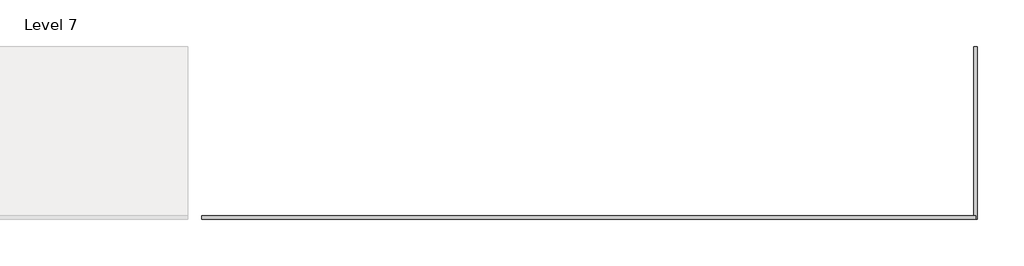
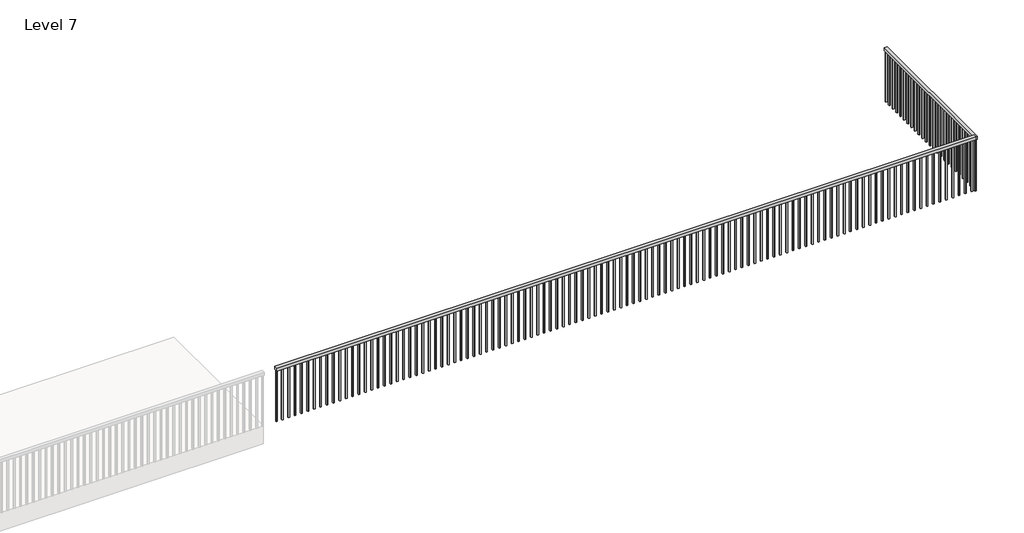
# One storey, part 2 of 5: 2 railings.
"""IFC4 building model written with IfcOpenShell, lengths in millimetres."""

from ifc_helpers import new_model, si_unit, frame, origin, place, context, project, spatial, polyline, outline, extrude, element, save

model = new_model("IFC4")

# Units and contexts
model_context = context("Model", 3, world=origin())
ifc_project = project(units=[si_unit("LENGTHUNIT", "METRE", prefix="MILLI")], contexts=[model_context])

# Site, building, storey
site = spatial("IfcSite", under=ifc_project)
building = spatial("IfcBuilding", under=site)
storey = spatial("IfcBuildingStorey", under=building, Name="Level 7", Elevation=6400.8)

# Railings
placement = place(None, origin())
element("IfcRailing", 1, ObjectType="Handrail - Rectangular", at=placement, inside=storey, context=model_context, shape_type="SweptSolid", body=[
    extrude(outline(polyline([(2981.3361222, -12911.7749501), (2981.3361222, -12860.9749501), (14106.5361222, -12860.9749501), (14106.5361222, -12911.7749501), (2981.3361222, -12911.7749501)])), frame((0.0, 0.0, 7264.4), z_axis=(0.0, 0.0, 1.0), x_axis=(1.0, 0.0, 0.0)), (0.0, 0.0, 1.0), 50.8),
    extrude(outline(polyline([(14046.2111222, -12895.8999501), (14046.2111222, -12876.8499501), (14065.2611222, -12876.8499501), (14065.2611222, -12895.8999501), (14046.2111222, -12895.8999501)])), frame((0.0, 0.0, 6400.8), z_axis=(0.0, 0.0, 1.0), x_axis=(1.0, 0.0, 0.0)), (0.0, 0.0, 1.0), 863.6),
    extrude(outline(polyline([(13944.6111222, -12895.8999501), (13944.6111222, -12876.8499501), (13963.6611222, -12876.8499501), (13963.6611222, -12895.8999501), (13944.6111222, -12895.8999501)])), frame((0.0, 0.0, 6400.8), z_axis=(0.0, 0.0, 1.0), x_axis=(1.0, 0.0, 0.0)), (0.0, 0.0, 1.0), 863.6),
    extrude(outline(polyline([(13843.0111222, -12895.8999501), (13843.0111222, -12876.8499501), (13862.0611222, -12876.8499501), (13862.0611222, -12895.8999501), (13843.0111222, -12895.8999501)])), frame((0.0, 0.0, 6400.8), z_axis=(0.0, 0.0, 1.0), x_axis=(1.0, 0.0, 0.0)), (0.0, 0.0, 1.0), 863.6),
    extrude(outline(polyline([(13741.4111222, -12895.8999501), (13741.4111222, -12876.8499501), (13760.4611222, -12876.8499501), (13760.4611222, -12895.8999501), (13741.4111222, -12895.8999501)])), frame((0.0, 0.0, 6400.8), z_axis=(0.0, 0.0, 1.0), x_axis=(1.0, 0.0, 0.0)), (0.0, 0.0, 1.0), 863.6),
    extrude(outline(polyline([(13639.8111222, -12895.8999501), (13639.8111222, -12876.8499501), (13658.8611222, -12876.8499501), (13658.8611222, -12895.8999501), (13639.8111222, -12895.8999501)])), frame((0.0, 0.0, 6400.8), z_axis=(0.0, 0.0, 1.0), x_axis=(1.0, 0.0, 0.0)), (0.0, 0.0, 1.0), 863.6),
    extrude(outline(polyline([(13538.2111222, -12895.8999501), (13538.2111222, -12876.8499501), (13557.2611222, -12876.8499501), (13557.2611222, -12895.8999501), (13538.2111222, -12895.8999501)])), frame((0.0, 0.0, 6400.8), z_axis=(0.0, 0.0, 1.0), x_axis=(1.0, 0.0, 0.0)), (0.0, 0.0, 1.0), 863.6),
    extrude(outline(polyline([(13436.6111222, -12895.8999501), (13436.6111222, -12876.8499501), (13455.6611222, -12876.8499501), (13455.6611222, -12895.8999501), (13436.6111222, -12895.8999501)])), frame((0.0, 0.0, 6400.8), z_axis=(0.0, 0.0, 1.0), x_axis=(1.0, 0.0, 0.0)), (0.0, 0.0, 1.0), 863.6),
    extrude(outline(polyline([(13335.0111222, -12895.8999501), (13335.0111222, -12876.8499501), (13354.0611222, -12876.8499501), (13354.0611222, -12895.8999501), (13335.0111222, -12895.8999501)])), frame((0.0, 0.0, 6400.8), z_axis=(0.0, 0.0, 1.0), x_axis=(1.0, 0.0, 0.0)), (0.0, 0.0, 1.0), 863.6),
    extrude(outline(polyline([(13233.4111222, -12895.8999501), (13233.4111222, -12876.8499501), (13252.4611222, -12876.8499501), (13252.4611222, -12895.8999501), (13233.4111222, -12895.8999501)])), frame((0.0, 0.0, 6400.8), z_axis=(0.0, 0.0, 1.0), x_axis=(1.0, 0.0, 0.0)), (0.0, 0.0, 1.0), 863.6),
    extrude(outline(polyline([(13131.8111222, -12895.8999501), (13131.8111222, -12876.8499501), (13150.8611222, -12876.8499501), (13150.8611222, -12895.8999501), (13131.8111222, -12895.8999501)])), frame((0.0, 0.0, 6400.8), z_axis=(0.0, 0.0, 1.0), x_axis=(1.0, 0.0, 0.0)), (0.0, 0.0, 1.0), 863.6),
    extrude(outline(polyline([(13030.2111222, -12895.8999501), (13030.2111222, -12876.8499501), (13049.2611222, -12876.8499501), (13049.2611222, -12895.8999501), (13030.2111222, -12895.8999501)])), frame((0.0, 0.0, 6400.8), z_axis=(0.0, 0.0, 1.0), x_axis=(1.0, 0.0, 0.0)), (0.0, 0.0, 1.0), 863.6),
    extrude(outline(polyline([(12928.6111222, -12895.8999501), (12928.6111222, -12876.8499501), (12947.6611222, -12876.8499501), (12947.6611222, -12895.8999501), (12928.6111222, -12895.8999501)])), frame((0.0, 0.0, 6400.8), z_axis=(0.0, 0.0, 1.0), x_axis=(1.0, 0.0, 0.0)), (0.0, 0.0, 1.0), 863.6),
    extrude(outline(polyline([(12827.0111222, -12895.8999501), (12827.0111222, -12876.8499501), (12846.0611222, -12876.8499501), (12846.0611222, -12895.8999501), (12827.0111222, -12895.8999501)])), frame((0.0, 0.0, 6400.8), z_axis=(0.0, 0.0, 1.0), x_axis=(1.0, 0.0, 0.0)), (0.0, 0.0, 1.0), 863.6),
    extrude(outline(polyline([(12725.4111222, -12895.8999501), (12725.4111222, -12876.8499501), (12744.4611222, -12876.8499501), (12744.4611222, -12895.8999501), (12725.4111222, -12895.8999501)])), frame((0.0, 0.0, 6400.8), z_axis=(0.0, 0.0, 1.0), x_axis=(1.0, 0.0, 0.0)), (0.0, 0.0, 1.0), 863.6),
    extrude(outline(polyline([(12623.8111222, -12895.8999501), (12623.8111222, -12876.8499501), (12642.8611222, -12876.8499501), (12642.8611222, -12895.8999501), (12623.8111222, -12895.8999501)])), frame((0.0, 0.0, 6400.8), z_axis=(0.0, 0.0, 1.0), x_axis=(1.0, 0.0, 0.0)), (0.0, 0.0, 1.0), 863.6),
    extrude(outline(polyline([(12522.2111222, -12895.8999501), (12522.2111222, -12876.8499501), (12541.2611222, -12876.8499501), (12541.2611222, -12895.8999501), (12522.2111222, -12895.8999501)])), frame((0.0, 0.0, 6400.8), z_axis=(0.0, 0.0, 1.0), x_axis=(1.0, 0.0, 0.0)), (0.0, 0.0, 1.0), 863.6),
    extrude(outline(polyline([(12420.6111222, -12895.8999501), (12420.6111222, -12876.8499501), (12439.6611222, -12876.8499501), (12439.6611222, -12895.8999501), (12420.6111222, -12895.8999501)])), frame((0.0, 0.0, 6400.8), z_axis=(0.0, 0.0, 1.0), x_axis=(1.0, 0.0, 0.0)), (0.0, 0.0, 1.0), 863.6),
    extrude(outline(polyline([(12319.0111222, -12895.8999501), (12319.0111222, -12876.8499501), (12338.0611222, -12876.8499501), (12338.0611222, -12895.8999501), (12319.0111222, -12895.8999501)])), frame((0.0, 0.0, 6400.8), z_axis=(0.0, 0.0, 1.0), x_axis=(1.0, 0.0, 0.0)), (0.0, 0.0, 1.0), 863.6),
    extrude(outline(polyline([(12217.4111222, -12895.8999501), (12217.4111222, -12876.8499501), (12236.4611222, -12876.8499501), (12236.4611222, -12895.8999501), (12217.4111222, -12895.8999501)])), frame((0.0, 0.0, 6400.8), z_axis=(0.0, 0.0, 1.0), x_axis=(1.0, 0.0, 0.0)), (0.0, 0.0, 1.0), 863.6),
    extrude(outline(polyline([(12115.8111222, -12895.8999501), (12115.8111222, -12876.8499501), (12134.8611222, -12876.8499501), (12134.8611222, -12895.8999501), (12115.8111222, -12895.8999501)])), frame((0.0, 0.0, 6400.8), z_axis=(0.0, 0.0, 1.0), x_axis=(1.0, 0.0, 0.0)), (0.0, 0.0, 1.0), 863.6),
    extrude(outline(polyline([(12014.2111222, -12895.8999501), (12014.2111222, -12876.8499501), (12033.2611222, -12876.8499501), (12033.2611222, -12895.8999501), (12014.2111222, -12895.8999501)])), frame((0.0, 0.0, 6400.8), z_axis=(0.0, 0.0, 1.0), x_axis=(1.0, 0.0, 0.0)), (0.0, 0.0, 1.0), 863.6),
    extrude(outline(polyline([(11912.6111222, -12895.8999501), (11912.6111222, -12876.8499501), (11931.6611222, -12876.8499501), (11931.6611222, -12895.8999501), (11912.6111222, -12895.8999501)])), frame((0.0, 0.0, 6400.8), z_axis=(0.0, 0.0, 1.0), x_axis=(1.0, 0.0, 0.0)), (0.0, 0.0, 1.0), 863.6),
    extrude(outline(polyline([(11811.0111222, -12895.8999501), (11811.0111222, -12876.8499501), (11830.0611222, -12876.8499501), (11830.0611222, -12895.8999501), (11811.0111222, -12895.8999501)])), frame((0.0, 0.0, 6400.8), z_axis=(0.0, 0.0, 1.0), x_axis=(1.0, 0.0, 0.0)), (0.0, 0.0, 1.0), 863.6),
    extrude(outline(polyline([(11709.4111222, -12895.8999501), (11709.4111222, -12876.8499501), (11728.4611222, -12876.8499501), (11728.4611222, -12895.8999501), (11709.4111222, -12895.8999501)])), frame((0.0, 0.0, 6400.8), z_axis=(0.0, 0.0, 1.0), x_axis=(1.0, 0.0, 0.0)), (0.0, 0.0, 1.0), 863.6),
    extrude(outline(polyline([(11607.8111222, -12895.8999501), (11607.8111222, -12876.8499501), (11626.8611222, -12876.8499501), (11626.8611222, -12895.8999501), (11607.8111222, -12895.8999501)])), frame((0.0, 0.0, 6400.8), z_axis=(0.0, 0.0, 1.0), x_axis=(1.0, 0.0, 0.0)), (0.0, 0.0, 1.0), 863.6),
    extrude(outline(polyline([(11506.2111222, -12895.8999501), (11506.2111222, -12876.8499501), (11525.2611222, -12876.8499501), (11525.2611222, -12895.8999501), (11506.2111222, -12895.8999501)])), frame((0.0, 0.0, 6400.8), z_axis=(0.0, 0.0, 1.0), x_axis=(1.0, 0.0, 0.0)), (0.0, 0.0, 1.0), 863.6),
    extrude(outline(polyline([(11404.6111222, -12895.8999501), (11404.6111222, -12876.8499501), (11423.6611222, -12876.8499501), (11423.6611222, -12895.8999501), (11404.6111222, -12895.8999501)])), frame((0.0, 0.0, 6400.8), z_axis=(0.0, 0.0, 1.0), x_axis=(1.0, 0.0, 0.0)), (0.0, 0.0, 1.0), 863.6),
    extrude(outline(polyline([(11303.0111222, -12895.8999501), (11303.0111222, -12876.8499501), (11322.0611222, -12876.8499501), (11322.0611222, -12895.8999501), (11303.0111222, -12895.8999501)])), frame((0.0, 0.0, 6400.8), z_axis=(0.0, 0.0, 1.0), x_axis=(1.0, 0.0, 0.0)), (0.0, 0.0, 1.0), 863.6),
    extrude(outline(polyline([(11201.4111222, -12895.8999501), (11201.4111222, -12876.8499501), (11220.4611222, -12876.8499501), (11220.4611222, -12895.8999501), (11201.4111222, -12895.8999501)])), frame((0.0, 0.0, 6400.8), z_axis=(0.0, 0.0, 1.0), x_axis=(1.0, 0.0, 0.0)), (0.0, 0.0, 1.0), 863.6),
    extrude(outline(polyline([(11099.8111222, -12895.8999501), (11099.8111222, -12876.8499501), (11118.8611222, -12876.8499501), (11118.8611222, -12895.8999501), (11099.8111222, -12895.8999501)])), frame((0.0, 0.0, 6400.8), z_axis=(0.0, 0.0, 1.0), x_axis=(1.0, 0.0, 0.0)), (0.0, 0.0, 1.0), 863.6),
    extrude(outline(polyline([(10998.2111222, -12895.8999501), (10998.2111222, -12876.8499501), (11017.2611222, -12876.8499501), (11017.2611222, -12895.8999501), (10998.2111222, -12895.8999501)])), frame((0.0, 0.0, 6400.8), z_axis=(0.0, 0.0, 1.0), x_axis=(1.0, 0.0, 0.0)), (0.0, 0.0, 1.0), 863.6),
    extrude(outline(polyline([(10896.6111222, -12895.8999501), (10896.6111222, -12876.8499501), (10915.6611222, -12876.8499501), (10915.6611222, -12895.8999501), (10896.6111222, -12895.8999501)])), frame((0.0, 0.0, 6400.8), z_axis=(0.0, 0.0, 1.0), x_axis=(1.0, 0.0, 0.0)), (0.0, 0.0, 1.0), 863.6),
    extrude(outline(polyline([(10795.0111222, -12895.8999501), (10795.0111222, -12876.8499501), (10814.0611222, -12876.8499501), (10814.0611222, -12895.8999501), (10795.0111222, -12895.8999501)])), frame((0.0, 0.0, 6400.8), z_axis=(0.0, 0.0, 1.0), x_axis=(1.0, 0.0, 0.0)), (0.0, 0.0, 1.0), 863.6),
    extrude(outline(polyline([(10693.4111222, -12895.8999501), (10693.4111222, -12876.8499501), (10712.4611222, -12876.8499501), (10712.4611222, -12895.8999501), (10693.4111222, -12895.8999501)])), frame((0.0, 0.0, 6400.8), z_axis=(0.0, 0.0, 1.0), x_axis=(1.0, 0.0, 0.0)), (0.0, 0.0, 1.0), 863.6),
    extrude(outline(polyline([(10591.8111222, -12895.8999501), (10591.8111222, -12876.8499501), (10610.8611222, -12876.8499501), (10610.8611222, -12895.8999501), (10591.8111222, -12895.8999501)])), frame((0.0, 0.0, 6400.8), z_axis=(0.0, 0.0, 1.0), x_axis=(1.0, 0.0, 0.0)), (0.0, 0.0, 1.0), 863.6),
    extrude(outline(polyline([(10490.2111222, -12895.8999501), (10490.2111222, -12876.8499501), (10509.2611222, -12876.8499501), (10509.2611222, -12895.8999501), (10490.2111222, -12895.8999501)])), frame((0.0, 0.0, 6400.8), z_axis=(0.0, 0.0, 1.0), x_axis=(1.0, 0.0, 0.0)), (0.0, 0.0, 1.0), 863.6),
    extrude(outline(polyline([(10388.6111222, -12895.8999501), (10388.6111222, -12876.8499501), (10407.6611222, -12876.8499501), (10407.6611222, -12895.8999501), (10388.6111222, -12895.8999501)])), frame((0.0, 0.0, 6400.8), z_axis=(0.0, 0.0, 1.0), x_axis=(1.0, 0.0, 0.0)), (0.0, 0.0, 1.0), 863.6),
    extrude(outline(polyline([(10287.0111222, -12895.8999501), (10287.0111222, -12876.8499501), (10306.0611222, -12876.8499501), (10306.0611222, -12895.8999501), (10287.0111222, -12895.8999501)])), frame((0.0, 0.0, 6400.8), z_axis=(0.0, 0.0, 1.0), x_axis=(1.0, 0.0, 0.0)), (0.0, 0.0, 1.0), 863.6),
    extrude(outline(polyline([(10185.4111222, -12895.8999501), (10185.4111222, -12876.8499501), (10204.4611222, -12876.8499501), (10204.4611222, -12895.8999501), (10185.4111222, -12895.8999501)])), frame((0.0, 0.0, 6400.8), z_axis=(0.0, 0.0, 1.0), x_axis=(1.0, 0.0, 0.0)), (0.0, 0.0, 1.0), 863.6),
    extrude(outline(polyline([(10083.8111222, -12895.8999501), (10083.8111222, -12876.8499501), (10102.8611222, -12876.8499501), (10102.8611222, -12895.8999501), (10083.8111222, -12895.8999501)])), frame((0.0, 0.0, 6400.8), z_axis=(0.0, 0.0, 1.0), x_axis=(1.0, 0.0, 0.0)), (0.0, 0.0, 1.0), 863.6),
    extrude(outline(polyline([(9982.2111222, -12895.8999501), (9982.2111222, -12876.8499501), (10001.2611222, -12876.8499501), (10001.2611222, -12895.8999501), (9982.2111222, -12895.8999501)])), frame((0.0, 0.0, 6400.8), z_axis=(0.0, 0.0, 1.0), x_axis=(1.0, 0.0, 0.0)), (0.0, 0.0, 1.0), 863.6),
    extrude(outline(polyline([(9880.6111222, -12895.8999501), (9880.6111222, -12876.8499501), (9899.6611222, -12876.8499501), (9899.6611222, -12895.8999501), (9880.6111222, -12895.8999501)])), frame((0.0, 0.0, 6400.8), z_axis=(0.0, 0.0, 1.0), x_axis=(1.0, 0.0, 0.0)), (0.0, 0.0, 1.0), 863.6),
    extrude(outline(polyline([(9779.0111222, -12895.8999501), (9779.0111222, -12876.8499501), (9798.0611222, -12876.8499501), (9798.0611222, -12895.8999501), (9779.0111222, -12895.8999501)])), frame((0.0, 0.0, 6400.8), z_axis=(0.0, 0.0, 1.0), x_axis=(1.0, 0.0, 0.0)), (0.0, 0.0, 1.0), 863.6),
    extrude(outline(polyline([(9677.4111222, -12895.8999501), (9677.4111222, -12876.8499501), (9696.4611222, -12876.8499501), (9696.4611222, -12895.8999501), (9677.4111222, -12895.8999501)])), frame((0.0, 0.0, 6400.8), z_axis=(0.0, 0.0, 1.0), x_axis=(1.0, 0.0, 0.0)), (0.0, 0.0, 1.0), 863.6),
    extrude(outline(polyline([(9575.8111222, -12895.8999501), (9575.8111222, -12876.8499501), (9594.8611222, -12876.8499501), (9594.8611222, -12895.8999501), (9575.8111222, -12895.8999501)])), frame((0.0, 0.0, 6400.8), z_axis=(0.0, 0.0, 1.0), x_axis=(1.0, 0.0, 0.0)), (0.0, 0.0, 1.0), 863.6),
    extrude(outline(polyline([(9474.2111222, -12895.8999501), (9474.2111222, -12876.8499501), (9493.2611222, -12876.8499501), (9493.2611222, -12895.8999501), (9474.2111222, -12895.8999501)])), frame((0.0, 0.0, 6400.8), z_axis=(0.0, 0.0, 1.0), x_axis=(1.0, 0.0, 0.0)), (0.0, 0.0, 1.0), 863.6),
    extrude(outline(polyline([(9372.6111222, -12895.8999501), (9372.6111222, -12876.8499501), (9391.6611222, -12876.8499501), (9391.6611222, -12895.8999501), (9372.6111222, -12895.8999501)])), frame((0.0, 0.0, 6400.8), z_axis=(0.0, 0.0, 1.0), x_axis=(1.0, 0.0, 0.0)), (0.0, 0.0, 1.0), 863.6),
    extrude(outline(polyline([(9271.0111222, -12895.8999501), (9271.0111222, -12876.8499501), (9290.0611222, -12876.8499501), (9290.0611222, -12895.8999501), (9271.0111222, -12895.8999501)])), frame((0.0, 0.0, 6400.8), z_axis=(0.0, 0.0, 1.0), x_axis=(1.0, 0.0, 0.0)), (0.0, 0.0, 1.0), 863.6),
    extrude(outline(polyline([(9169.4111222, -12895.8999501), (9169.4111222, -12876.8499501), (9188.4611222, -12876.8499501), (9188.4611222, -12895.8999501), (9169.4111222, -12895.8999501)])), frame((0.0, 0.0, 6400.8), z_axis=(0.0, 0.0, 1.0), x_axis=(1.0, 0.0, 0.0)), (0.0, 0.0, 1.0), 863.6),
    extrude(outline(polyline([(9067.8111222, -12895.8999501), (9067.8111222, -12876.8499501), (9086.8611222, -12876.8499501), (9086.8611222, -12895.8999501), (9067.8111222, -12895.8999501)])), frame((0.0, 0.0, 6400.8), z_axis=(0.0, 0.0, 1.0), x_axis=(1.0, 0.0, 0.0)), (0.0, 0.0, 1.0), 863.6),
    extrude(outline(polyline([(8966.2111222, -12895.8999501), (8966.2111222, -12876.8499501), (8985.2611222, -12876.8499501), (8985.2611222, -12895.8999501), (8966.2111222, -12895.8999501)])), frame((0.0, 0.0, 6400.8), z_axis=(0.0, 0.0, 1.0), x_axis=(1.0, 0.0, 0.0)), (0.0, 0.0, 1.0), 863.6),
    extrude(outline(polyline([(8864.6111222, -12895.8999501), (8864.6111222, -12876.8499501), (8883.6611222, -12876.8499501), (8883.6611222, -12895.8999501), (8864.6111222, -12895.8999501)])), frame((0.0, 0.0, 6400.8), z_axis=(0.0, 0.0, 1.0), x_axis=(1.0, 0.0, 0.0)), (0.0, 0.0, 1.0), 863.6),
    extrude(outline(polyline([(8763.0111222, -12895.8999501), (8763.0111222, -12876.8499501), (8782.0611222, -12876.8499501), (8782.0611222, -12895.8999501), (8763.0111222, -12895.8999501)])), frame((0.0, 0.0, 6400.8), z_axis=(0.0, 0.0, 1.0), x_axis=(1.0, 0.0, 0.0)), (0.0, 0.0, 1.0), 863.6),
    extrude(outline(polyline([(8661.4111222, -12895.8999501), (8661.4111222, -12876.8499501), (8680.4611222, -12876.8499501), (8680.4611222, -12895.8999501), (8661.4111222, -12895.8999501)])), frame((0.0, 0.0, 6400.8), z_axis=(0.0, 0.0, 1.0), x_axis=(1.0, 0.0, 0.0)), (0.0, 0.0, 1.0), 863.6),
    extrude(outline(polyline([(8559.8111222, -12895.8999501), (8559.8111222, -12876.8499501), (8578.8611222, -12876.8499501), (8578.8611222, -12895.8999501), (8559.8111222, -12895.8999501)])), frame((0.0, 0.0, 6400.8), z_axis=(0.0, 0.0, 1.0), x_axis=(1.0, 0.0, 0.0)), (0.0, 0.0, 1.0), 863.6),
    extrude(outline(polyline([(8458.2111222, -12895.8999501), (8458.2111222, -12876.8499501), (8477.2611222, -12876.8499501), (8477.2611222, -12895.8999501), (8458.2111222, -12895.8999501)])), frame((0.0, 0.0, 6400.8), z_axis=(0.0, 0.0, 1.0), x_axis=(1.0, 0.0, 0.0)), (0.0, 0.0, 1.0), 863.6),
    extrude(outline(polyline([(8356.6111222, -12895.8999501), (8356.6111222, -12876.8499501), (8375.6611222, -12876.8499501), (8375.6611222, -12895.8999501), (8356.6111222, -12895.8999501)])), frame((0.0, 0.0, 6400.8), z_axis=(0.0, 0.0, 1.0), x_axis=(1.0, 0.0, 0.0)), (0.0, 0.0, 1.0), 863.6),
    extrude(outline(polyline([(8255.0111222, -12895.8999501), (8255.0111222, -12876.8499501), (8274.0611222, -12876.8499501), (8274.0611222, -12895.8999501), (8255.0111222, -12895.8999501)])), frame((0.0, 0.0, 6400.8), z_axis=(0.0, 0.0, 1.0), x_axis=(1.0, 0.0, 0.0)), (0.0, 0.0, 1.0), 863.6),
    extrude(outline(polyline([(8153.4111222, -12895.8999501), (8153.4111222, -12876.8499501), (8172.4611222, -12876.8499501), (8172.4611222, -12895.8999501), (8153.4111222, -12895.8999501)])), frame((0.0, 0.0, 6400.8), z_axis=(0.0, 0.0, 1.0), x_axis=(1.0, 0.0, 0.0)), (0.0, 0.0, 1.0), 863.6),
    extrude(outline(polyline([(8051.8111222, -12895.8999501), (8051.8111222, -12876.8499501), (8070.8611222, -12876.8499501), (8070.8611222, -12895.8999501), (8051.8111222, -12895.8999501)])), frame((0.0, 0.0, 6400.8), z_axis=(0.0, 0.0, 1.0), x_axis=(1.0, 0.0, 0.0)), (0.0, 0.0, 1.0), 863.6),
    extrude(outline(polyline([(7950.2111222, -12895.8999501), (7950.2111222, -12876.8499501), (7969.2611222, -12876.8499501), (7969.2611222, -12895.8999501), (7950.2111222, -12895.8999501)])), frame((0.0, 0.0, 6400.8), z_axis=(0.0, 0.0, 1.0), x_axis=(1.0, 0.0, 0.0)), (0.0, 0.0, 1.0), 863.6),
    extrude(outline(polyline([(7848.6111222, -12895.8999501), (7848.6111222, -12876.8499501), (7867.6611222, -12876.8499501), (7867.6611222, -12895.8999501), (7848.6111222, -12895.8999501)])), frame((0.0, 0.0, 6400.8), z_axis=(0.0, 0.0, 1.0), x_axis=(1.0, 0.0, 0.0)), (0.0, 0.0, 1.0), 863.6),
    extrude(outline(polyline([(7747.0111222, -12895.8999501), (7747.0111222, -12876.8499501), (7766.0611222, -12876.8499501), (7766.0611222, -12895.8999501), (7747.0111222, -12895.8999501)])), frame((0.0, 0.0, 6400.8), z_axis=(0.0, 0.0, 1.0), x_axis=(1.0, 0.0, 0.0)), (0.0, 0.0, 1.0), 863.6),
    extrude(outline(polyline([(7645.4111222, -12895.8999501), (7645.4111222, -12876.8499501), (7664.4611222, -12876.8499501), (7664.4611222, -12895.8999501), (7645.4111222, -12895.8999501)])), frame((0.0, 0.0, 6400.8), z_axis=(0.0, 0.0, 1.0), x_axis=(1.0, 0.0, 0.0)), (0.0, 0.0, 1.0), 863.6),
    extrude(outline(polyline([(7543.8111222, -12895.8999501), (7543.8111222, -12876.8499501), (7562.8611222, -12876.8499501), (7562.8611222, -12895.8999501), (7543.8111222, -12895.8999501)])), frame((0.0, 0.0, 6400.8), z_axis=(0.0, 0.0, 1.0), x_axis=(1.0, 0.0, 0.0)), (0.0, 0.0, 1.0), 863.6),
    extrude(outline(polyline([(7442.2111222, -12895.8999501), (7442.2111222, -12876.8499501), (7461.2611222, -12876.8499501), (7461.2611222, -12895.8999501), (7442.2111222, -12895.8999501)])), frame((0.0, 0.0, 6400.8), z_axis=(0.0, 0.0, 1.0), x_axis=(1.0, 0.0, 0.0)), (0.0, 0.0, 1.0), 863.6),
    extrude(outline(polyline([(7340.6111222, -12895.8999501), (7340.6111222, -12876.8499501), (7359.6611222, -12876.8499501), (7359.6611222, -12895.8999501), (7340.6111222, -12895.8999501)])), frame((0.0, 0.0, 6400.8), z_axis=(0.0, 0.0, 1.0), x_axis=(1.0, 0.0, 0.0)), (0.0, 0.0, 1.0), 863.6),
    extrude(outline(polyline([(7239.0111222, -12895.8999501), (7239.0111222, -12876.8499501), (7258.0611222, -12876.8499501), (7258.0611222, -12895.8999501), (7239.0111222, -12895.8999501)])), frame((0.0, 0.0, 6400.8), z_axis=(0.0, 0.0, 1.0), x_axis=(1.0, 0.0, 0.0)), (0.0, 0.0, 1.0), 863.6),
    extrude(outline(polyline([(7137.4111222, -12895.8999501), (7137.4111222, -12876.8499501), (7156.4611222, -12876.8499501), (7156.4611222, -12895.8999501), (7137.4111222, -12895.8999501)])), frame((0.0, 0.0, 6400.8), z_axis=(0.0, 0.0, 1.0), x_axis=(1.0, 0.0, 0.0)), (0.0, 0.0, 1.0), 863.6),
    extrude(outline(polyline([(7035.8111222, -12895.8999501), (7035.8111222, -12876.8499501), (7054.8611222, -12876.8499501), (7054.8611222, -12895.8999501), (7035.8111222, -12895.8999501)])), frame((0.0, 0.0, 6400.8), z_axis=(0.0, 0.0, 1.0), x_axis=(1.0, 0.0, 0.0)), (0.0, 0.0, 1.0), 863.6),
    extrude(outline(polyline([(6934.2111222, -12895.8999501), (6934.2111222, -12876.8499501), (6953.2611222, -12876.8499501), (6953.2611222, -12895.8999501), (6934.2111222, -12895.8999501)])), frame((0.0, 0.0, 6400.8), z_axis=(0.0, 0.0, 1.0), x_axis=(1.0, 0.0, 0.0)), (0.0, 0.0, 1.0), 863.6),
    extrude(outline(polyline([(6832.6111222, -12895.8999501), (6832.6111222, -12876.8499501), (6851.6611222, -12876.8499501), (6851.6611222, -12895.8999501), (6832.6111222, -12895.8999501)])), frame((0.0, 0.0, 6400.8), z_axis=(0.0, 0.0, 1.0), x_axis=(1.0, 0.0, 0.0)), (0.0, 0.0, 1.0), 863.6),
    extrude(outline(polyline([(6731.0111222, -12895.8999501), (6731.0111222, -12876.8499501), (6750.0611222, -12876.8499501), (6750.0611222, -12895.8999501), (6731.0111222, -12895.8999501)])), frame((0.0, 0.0, 6400.8), z_axis=(0.0, 0.0, 1.0), x_axis=(1.0, 0.0, 0.0)), (0.0, 0.0, 1.0), 863.6),
    extrude(outline(polyline([(6629.4111222, -12895.8999501), (6629.4111222, -12876.8499501), (6648.4611222, -12876.8499501), (6648.4611222, -12895.8999501), (6629.4111222, -12895.8999501)])), frame((0.0, 0.0, 6400.8), z_axis=(0.0, 0.0, 1.0), x_axis=(1.0, 0.0, 0.0)), (0.0, 0.0, 1.0), 863.6),
    extrude(outline(polyline([(6527.8111222, -12895.8999501), (6527.8111222, -12876.8499501), (6546.8611222, -12876.8499501), (6546.8611222, -12895.8999501), (6527.8111222, -12895.8999501)])), frame((0.0, 0.0, 6400.8), z_axis=(0.0, 0.0, 1.0), x_axis=(1.0, 0.0, 0.0)), (0.0, 0.0, 1.0), 863.6),
    extrude(outline(polyline([(6426.2111222, -12895.8999501), (6426.2111222, -12876.8499501), (6445.2611222, -12876.8499501), (6445.2611222, -12895.8999501), (6426.2111222, -12895.8999501)])), frame((0.0, 0.0, 6400.8), z_axis=(0.0, 0.0, 1.0), x_axis=(1.0, 0.0, 0.0)), (0.0, 0.0, 1.0), 863.6),
    extrude(outline(polyline([(6324.6111222, -12895.8999501), (6324.6111222, -12876.8499501), (6343.6611222, -12876.8499501), (6343.6611222, -12895.8999501), (6324.6111222, -12895.8999501)])), frame((0.0, 0.0, 6400.8), z_axis=(0.0, 0.0, 1.0), x_axis=(1.0, 0.0, 0.0)), (0.0, 0.0, 1.0), 863.6),
    extrude(outline(polyline([(6223.0111222, -12895.8999501), (6223.0111222, -12876.8499501), (6242.0611222, -12876.8499501), (6242.0611222, -12895.8999501), (6223.0111222, -12895.8999501)])), frame((0.0, 0.0, 6400.8), z_axis=(0.0, 0.0, 1.0), x_axis=(1.0, 0.0, 0.0)), (0.0, 0.0, 1.0), 863.6),
    extrude(outline(polyline([(6121.4111222, -12895.8999501), (6121.4111222, -12876.8499501), (6140.4611222, -12876.8499501), (6140.4611222, -12895.8999501), (6121.4111222, -12895.8999501)])), frame((0.0, 0.0, 6400.8), z_axis=(0.0, 0.0, 1.0), x_axis=(1.0, 0.0, 0.0)), (0.0, 0.0, 1.0), 863.6),
    extrude(outline(polyline([(6019.8111222, -12895.8999501), (6019.8111222, -12876.8499501), (6038.8611222, -12876.8499501), (6038.8611222, -12895.8999501), (6019.8111222, -12895.8999501)])), frame((0.0, 0.0, 6400.8), z_axis=(0.0, 0.0, 1.0), x_axis=(1.0, 0.0, 0.0)), (0.0, 0.0, 1.0), 863.6),
    extrude(outline(polyline([(5918.2111222, -12895.8999501), (5918.2111222, -12876.8499501), (5937.2611222, -12876.8499501), (5937.2611222, -12895.8999501), (5918.2111222, -12895.8999501)])), frame((0.0, 0.0, 6400.8), z_axis=(0.0, 0.0, 1.0), x_axis=(1.0, 0.0, 0.0)), (0.0, 0.0, 1.0), 863.6),
    extrude(outline(polyline([(5816.6111222, -12895.8999501), (5816.6111222, -12876.8499501), (5835.6611222, -12876.8499501), (5835.6611222, -12895.8999501), (5816.6111222, -12895.8999501)])), frame((0.0, 0.0, 6400.8), z_axis=(0.0, 0.0, 1.0), x_axis=(1.0, 0.0, 0.0)), (0.0, 0.0, 1.0), 863.6),
    extrude(outline(polyline([(5715.0111222, -12895.8999501), (5715.0111222, -12876.8499501), (5734.0611222, -12876.8499501), (5734.0611222, -12895.8999501), (5715.0111222, -12895.8999501)])), frame((0.0, 0.0, 6400.8), z_axis=(0.0, 0.0, 1.0), x_axis=(1.0, 0.0, 0.0)), (0.0, 0.0, 1.0), 863.6),
    extrude(outline(polyline([(5613.4111222, -12895.8999501), (5613.4111222, -12876.8499501), (5632.4611222, -12876.8499501), (5632.4611222, -12895.8999501), (5613.4111222, -12895.8999501)])), frame((0.0, 0.0, 6400.8), z_axis=(0.0, 0.0, 1.0), x_axis=(1.0, 0.0, 0.0)), (0.0, 0.0, 1.0), 863.6),
    extrude(outline(polyline([(5511.8111222, -12895.8999501), (5511.8111222, -12876.8499501), (5530.8611222, -12876.8499501), (5530.8611222, -12895.8999501), (5511.8111222, -12895.8999501)])), frame((0.0, 0.0, 6400.8), z_axis=(0.0, 0.0, 1.0), x_axis=(1.0, 0.0, 0.0)), (0.0, 0.0, 1.0), 863.6),
    extrude(outline(polyline([(5410.2111222, -12895.8999501), (5410.2111222, -12876.8499501), (5429.2611222, -12876.8499501), (5429.2611222, -12895.8999501), (5410.2111222, -12895.8999501)])), frame((0.0, 0.0, 6400.8), z_axis=(0.0, 0.0, 1.0), x_axis=(1.0, 0.0, 0.0)), (0.0, 0.0, 1.0), 863.6),
    extrude(outline(polyline([(5308.6111222, -12895.8999501), (5308.6111222, -12876.8499501), (5327.6611222, -12876.8499501), (5327.6611222, -12895.8999501), (5308.6111222, -12895.8999501)])), frame((0.0, 0.0, 6400.8), z_axis=(0.0, 0.0, 1.0), x_axis=(1.0, 0.0, 0.0)), (0.0, 0.0, 1.0), 863.6),
    extrude(outline(polyline([(5207.0111222, -12895.8999501), (5207.0111222, -12876.8499501), (5226.0611222, -12876.8499501), (5226.0611222, -12895.8999501), (5207.0111222, -12895.8999501)])), frame((0.0, 0.0, 6400.8), z_axis=(0.0, 0.0, 1.0), x_axis=(1.0, 0.0, 0.0)), (0.0, 0.0, 1.0), 863.6),
    extrude(outline(polyline([(5105.4111222, -12895.8999501), (5105.4111222, -12876.8499501), (5124.4611222, -12876.8499501), (5124.4611222, -12895.8999501), (5105.4111222, -12895.8999501)])), frame((0.0, 0.0, 6400.8), z_axis=(0.0, 0.0, 1.0), x_axis=(1.0, 0.0, 0.0)), (0.0, 0.0, 1.0), 863.6),
    extrude(outline(polyline([(5003.8111222, -12895.8999501), (5003.8111222, -12876.8499501), (5022.8611222, -12876.8499501), (5022.8611222, -12895.8999501), (5003.8111222, -12895.8999501)])), frame((0.0, 0.0, 6400.8), z_axis=(0.0, 0.0, 1.0), x_axis=(1.0, 0.0, 0.0)), (0.0, 0.0, 1.0), 863.6),
    extrude(outline(polyline([(4902.2111222, -12895.8999501), (4902.2111222, -12876.8499501), (4921.2611222, -12876.8499501), (4921.2611222, -12895.8999501), (4902.2111222, -12895.8999501)])), frame((0.0, 0.0, 6400.8), z_axis=(0.0, 0.0, 1.0), x_axis=(1.0, 0.0, 0.0)), (0.0, 0.0, 1.0), 863.6),
    extrude(outline(polyline([(4800.6111222, -12895.8999501), (4800.6111222, -12876.8499501), (4819.6611222, -12876.8499501), (4819.6611222, -12895.8999501), (4800.6111222, -12895.8999501)])), frame((0.0, 0.0, 6400.8), z_axis=(0.0, 0.0, 1.0), x_axis=(1.0, 0.0, 0.0)), (0.0, 0.0, 1.0), 863.6),
    extrude(outline(polyline([(4699.0111222, -12895.8999501), (4699.0111222, -12876.8499501), (4718.0611222, -12876.8499501), (4718.0611222, -12895.8999501), (4699.0111222, -12895.8999501)])), frame((0.0, 0.0, 6400.8), z_axis=(0.0, 0.0, 1.0), x_axis=(1.0, 0.0, 0.0)), (0.0, 0.0, 1.0), 863.6),
    extrude(outline(polyline([(4597.4111222, -12895.8999501), (4597.4111222, -12876.8499501), (4616.4611222, -12876.8499501), (4616.4611222, -12895.8999501), (4597.4111222, -12895.8999501)])), frame((0.0, 0.0, 6400.8), z_axis=(0.0, 0.0, 1.0), x_axis=(1.0, 0.0, 0.0)), (0.0, 0.0, 1.0), 863.6),
    extrude(outline(polyline([(4495.8111222, -12895.8999501), (4495.8111222, -12876.8499501), (4514.8611222, -12876.8499501), (4514.8611222, -12895.8999501), (4495.8111222, -12895.8999501)])), frame((0.0, 0.0, 6400.8), z_axis=(0.0, 0.0, 1.0), x_axis=(1.0, 0.0, 0.0)), (0.0, 0.0, 1.0), 863.6),
    extrude(outline(polyline([(4394.2111222, -12895.8999501), (4394.2111222, -12876.8499501), (4413.2611222, -12876.8499501), (4413.2611222, -12895.8999501), (4394.2111222, -12895.8999501)])), frame((0.0, 0.0, 6400.8), z_axis=(0.0, 0.0, 1.0), x_axis=(1.0, 0.0, 0.0)), (0.0, 0.0, 1.0), 863.6),
    extrude(outline(polyline([(4292.6111222, -12895.8999501), (4292.6111222, -12876.8499501), (4311.6611222, -12876.8499501), (4311.6611222, -12895.8999501), (4292.6111222, -12895.8999501)])), frame((0.0, 0.0, 6400.8), z_axis=(0.0, 0.0, 1.0), x_axis=(1.0, 0.0, 0.0)), (0.0, 0.0, 1.0), 863.6),
    extrude(outline(polyline([(4191.0111222, -12895.8999501), (4191.0111222, -12876.8499501), (4210.0611222, -12876.8499501), (4210.0611222, -12895.8999501), (4191.0111222, -12895.8999501)])), frame((0.0, 0.0, 6400.8), z_axis=(0.0, 0.0, 1.0), x_axis=(1.0, 0.0, 0.0)), (0.0, 0.0, 1.0), 863.6),
    extrude(outline(polyline([(4089.4111222, -12895.8999501), (4089.4111222, -12876.8499501), (4108.4611222, -12876.8499501), (4108.4611222, -12895.8999501), (4089.4111222, -12895.8999501)])), frame((0.0, 0.0, 6400.8), z_axis=(0.0, 0.0, 1.0), x_axis=(1.0, 0.0, 0.0)), (0.0, 0.0, 1.0), 863.6),
    extrude(outline(polyline([(3987.8111222, -12895.8999501), (3987.8111222, -12876.8499501), (4006.8611222, -12876.8499501), (4006.8611222, -12895.8999501), (3987.8111222, -12895.8999501)])), frame((0.0, 0.0, 6400.8), z_axis=(0.0, 0.0, 1.0), x_axis=(1.0, 0.0, 0.0)), (0.0, 0.0, 1.0), 863.6),
    extrude(outline(polyline([(3886.2111222, -12895.8999501), (3886.2111222, -12876.8499501), (3905.2611222, -12876.8499501), (3905.2611222, -12895.8999501), (3886.2111222, -12895.8999501)])), frame((0.0, 0.0, 6400.8), z_axis=(0.0, 0.0, 1.0), x_axis=(1.0, 0.0, 0.0)), (0.0, 0.0, 1.0), 863.6),
    extrude(outline(polyline([(3784.6111222, -12895.8999501), (3784.6111222, -12876.8499501), (3803.6611222, -12876.8499501), (3803.6611222, -12895.8999501), (3784.6111222, -12895.8999501)])), frame((0.0, 0.0, 6400.8), z_axis=(0.0, 0.0, 1.0), x_axis=(1.0, 0.0, 0.0)), (0.0, 0.0, 1.0), 863.6),
    extrude(outline(polyline([(3683.0111222, -12895.8999501), (3683.0111222, -12876.8499501), (3702.0611222, -12876.8499501), (3702.0611222, -12895.8999501), (3683.0111222, -12895.8999501)])), frame((0.0, 0.0, 6400.8), z_axis=(0.0, 0.0, 1.0), x_axis=(1.0, 0.0, 0.0)), (0.0, 0.0, 1.0), 863.6),
    extrude(outline(polyline([(3581.4111222, -12895.8999501), (3581.4111222, -12876.8499501), (3600.4611222, -12876.8499501), (3600.4611222, -12895.8999501), (3581.4111222, -12895.8999501)])), frame((0.0, 0.0, 6400.8), z_axis=(0.0, 0.0, 1.0), x_axis=(1.0, 0.0, 0.0)), (0.0, 0.0, 1.0), 863.6),
    extrude(outline(polyline([(3479.8111222, -12895.8999501), (3479.8111222, -12876.8499501), (3498.8611222, -12876.8499501), (3498.8611222, -12895.8999501), (3479.8111222, -12895.8999501)])), frame((0.0, 0.0, 6400.8), z_axis=(0.0, 0.0, 1.0), x_axis=(1.0, 0.0, 0.0)), (0.0, 0.0, 1.0), 863.6),
    extrude(outline(polyline([(3378.2111222, -12895.8999501), (3378.2111222, -12876.8499501), (3397.2611222, -12876.8499501), (3397.2611222, -12895.8999501), (3378.2111222, -12895.8999501)])), frame((0.0, 0.0, 6400.8), z_axis=(0.0, 0.0, 1.0), x_axis=(1.0, 0.0, 0.0)), (0.0, 0.0, 1.0), 863.6),
    extrude(outline(polyline([(3276.6111222, -12895.8999501), (3276.6111222, -12876.8499501), (3295.6611222, -12876.8499501), (3295.6611222, -12895.8999501), (3276.6111222, -12895.8999501)])), frame((0.0, 0.0, 6400.8), z_axis=(0.0, 0.0, 1.0), x_axis=(1.0, 0.0, 0.0)), (0.0, 0.0, 1.0), 863.6),
    extrude(outline(polyline([(3175.0111222, -12895.8999501), (3175.0111222, -12876.8499501), (3194.0611222, -12876.8499501), (3194.0611222, -12895.8999501), (3175.0111222, -12895.8999501)])), frame((0.0, 0.0, 6400.8), z_axis=(0.0, 0.0, 1.0), x_axis=(1.0, 0.0, 0.0)), (0.0, 0.0, 1.0), 863.6),
    extrude(outline(polyline([(3073.4111222, -12895.8999501), (3073.4111222, -12876.8499501), (3092.4611222, -12876.8499501), (3092.4611222, -12895.8999501), (3073.4111222, -12895.8999501)])), frame((0.0, 0.0, 6400.8), z_axis=(0.0, 0.0, 1.0), x_axis=(1.0, 0.0, 0.0)), (0.0, 0.0, 1.0), 863.6),
    extrude(outline(polyline([(14087.4861222, -12895.8999501), (14087.4861222, -12876.8499501), (14106.5361222, -12876.8499501), (14106.5361222, -12895.8999501), (14087.4861222, -12895.8999501)])), frame((0.0, 0.0, 6400.8), z_axis=(0.0, 0.0, 1.0), x_axis=(1.0, 0.0, 0.0)), (0.0, 0.0, 1.0), 863.6),
    extrude(outline(polyline([(2981.3361222, -12895.8999501), (2981.3361222, -12876.8499501), (3000.3861222, -12876.8499501), (3000.3861222, -12895.8999501), (2981.3361222, -12895.8999501)])), frame((0.0, 0.0, 6400.8), z_axis=(0.0, 0.0, 1.0), x_axis=(1.0, 0.0, 0.0)), (0.0, 0.0, 1.0), 863.6),
])
element("IfcRailing", 2, ObjectType="Handrail - Rectangular", at=placement, inside=storey, context=model_context, shape_type="SweptSolid", body=[
    extrude(outline(polyline([(14081.1361222, -10428.1762475), (14131.9361222, -10428.1762475), (14131.9361222, -12911.7749501), (14081.1361222, -12911.7749501), (14081.1361222, -10428.1762475)])), frame((0.0, 0.0, 7264.4), z_axis=(0.0, 0.0, 1.0), x_axis=(1.0, 0.0, 0.0)), (0.0, 0.0, 1.0), 50.8),
    extrude(outline(polyline([(14097.0111222, -12857.0512475), (14116.0611222, -12857.0512475), (14116.0611222, -12876.1012475), (14097.0111222, -12876.1012475), (14097.0111222, -12857.0512475)])), frame((0.0, 0.0, 6400.8), z_axis=(0.0, 0.0, 1.0), x_axis=(1.0, 0.0, 0.0)), (0.0, 0.0, 1.0), 863.6),
    extrude(outline(polyline([(14097.0111222, -12755.4512475), (14116.0611222, -12755.4512475), (14116.0611222, -12774.5012475), (14097.0111222, -12774.5012475), (14097.0111222, -12755.4512475)])), frame((0.0, 0.0, 6400.8), z_axis=(0.0, 0.0, 1.0), x_axis=(1.0, 0.0, 0.0)), (0.0, 0.0, 1.0), 863.6),
    extrude(outline(polyline([(14097.0111222, -12653.8512475), (14116.0611222, -12653.8512475), (14116.0611222, -12672.9012475), (14097.0111222, -12672.9012475), (14097.0111222, -12653.8512475)])), frame((0.0, 0.0, 6400.8), z_axis=(0.0, 0.0, 1.0), x_axis=(1.0, 0.0, 0.0)), (0.0, 0.0, 1.0), 863.6),
    extrude(outline(polyline([(14097.0111222, -12552.2512475), (14116.0611222, -12552.2512475), (14116.0611222, -12571.3012475), (14097.0111222, -12571.3012475), (14097.0111222, -12552.2512475)])), frame((0.0, 0.0, 6400.8), z_axis=(0.0, 0.0, 1.0), x_axis=(1.0, 0.0, 0.0)), (0.0, 0.0, 1.0), 863.6),
    extrude(outline(polyline([(14097.0111222, -12450.6512475), (14116.0611222, -12450.6512475), (14116.0611222, -12469.7012475), (14097.0111222, -12469.7012475), (14097.0111222, -12450.6512475)])), frame((0.0, 0.0, 6400.8), z_axis=(0.0, 0.0, 1.0), x_axis=(1.0, 0.0, 0.0)), (0.0, 0.0, 1.0), 863.6),
    extrude(outline(polyline([(14097.0111222, -12349.0512475), (14116.0611222, -12349.0512475), (14116.0611222, -12368.1012475), (14097.0111222, -12368.1012475), (14097.0111222, -12349.0512475)])), frame((0.0, 0.0, 6400.8), z_axis=(0.0, 0.0, 1.0), x_axis=(1.0, 0.0, 0.0)), (0.0, 0.0, 1.0), 863.6),
    extrude(outline(polyline([(14097.0111222, -12247.4512475), (14116.0611222, -12247.4512475), (14116.0611222, -12266.5012475), (14097.0111222, -12266.5012475), (14097.0111222, -12247.4512475)])), frame((0.0, 0.0, 6400.8), z_axis=(0.0, 0.0, 1.0), x_axis=(1.0, 0.0, 0.0)), (0.0, 0.0, 1.0), 863.6),
    extrude(outline(polyline([(14097.0111222, -12145.8512475), (14116.0611222, -12145.8512475), (14116.0611222, -12164.9012475), (14097.0111222, -12164.9012475), (14097.0111222, -12145.8512475)])), frame((0.0, 0.0, 6400.8), z_axis=(0.0, 0.0, 1.0), x_axis=(1.0, 0.0, 0.0)), (0.0, 0.0, 1.0), 863.6),
    extrude(outline(polyline([(14097.0111222, -12044.2512475), (14116.0611222, -12044.2512475), (14116.0611222, -12063.3012475), (14097.0111222, -12063.3012475), (14097.0111222, -12044.2512475)])), frame((0.0, 0.0, 6400.8), z_axis=(0.0, 0.0, 1.0), x_axis=(1.0, 0.0, 0.0)), (0.0, 0.0, 1.0), 863.6),
    extrude(outline(polyline([(14097.0111222, -11942.6512475), (14116.0611222, -11942.6512475), (14116.0611222, -11961.7012475), (14097.0111222, -11961.7012475), (14097.0111222, -11942.6512475)])), frame((0.0, 0.0, 6400.8), z_axis=(0.0, 0.0, 1.0), x_axis=(1.0, 0.0, 0.0)), (0.0, 0.0, 1.0), 863.6),
    extrude(outline(polyline([(14097.0111222, -11841.0512475), (14116.0611222, -11841.0512475), (14116.0611222, -11860.1012475), (14097.0111222, -11860.1012475), (14097.0111222, -11841.0512475)])), frame((0.0, 0.0, 6400.8), z_axis=(0.0, 0.0, 1.0), x_axis=(1.0, 0.0, 0.0)), (0.0, 0.0, 1.0), 863.6),
    extrude(outline(polyline([(14097.0111222, -11739.4512475), (14116.0611222, -11739.4512475), (14116.0611222, -11758.5012475), (14097.0111222, -11758.5012475), (14097.0111222, -11739.4512475)])), frame((0.0, 0.0, 6400.8), z_axis=(0.0, 0.0, 1.0), x_axis=(1.0, 0.0, 0.0)), (0.0, 0.0, 1.0), 863.6),
    extrude(outline(polyline([(14097.0111222, -11637.8512475), (14116.0611222, -11637.8512475), (14116.0611222, -11656.9012475), (14097.0111222, -11656.9012475), (14097.0111222, -11637.8512475)])), frame((0.0, 0.0, 6400.8), z_axis=(0.0, 0.0, 1.0), x_axis=(1.0, 0.0, 0.0)), (0.0, 0.0, 1.0), 863.6),
    extrude(outline(polyline([(14097.0111222, -11536.2512475), (14116.0611222, -11536.2512475), (14116.0611222, -11555.3012475), (14097.0111222, -11555.3012475), (14097.0111222, -11536.2512475)])), frame((0.0, 0.0, 6400.8), z_axis=(0.0, 0.0, 1.0), x_axis=(1.0, 0.0, 0.0)), (0.0, 0.0, 1.0), 863.6),
    extrude(outline(polyline([(14097.0111222, -11434.6512475), (14116.0611222, -11434.6512475), (14116.0611222, -11453.7012475), (14097.0111222, -11453.7012475), (14097.0111222, -11434.6512475)])), frame((0.0, 0.0, 6400.8), z_axis=(0.0, 0.0, 1.0), x_axis=(1.0, 0.0, 0.0)), (0.0, 0.0, 1.0), 863.6),
    extrude(outline(polyline([(14097.0111222, -11333.0512475), (14116.0611222, -11333.0512475), (14116.0611222, -11352.1012475), (14097.0111222, -11352.1012475), (14097.0111222, -11333.0512475)])), frame((0.0, 0.0, 6400.8), z_axis=(0.0, 0.0, 1.0), x_axis=(1.0, 0.0, 0.0)), (0.0, 0.0, 1.0), 863.6),
    extrude(outline(polyline([(14097.0111222, -11231.4512475), (14116.0611222, -11231.4512475), (14116.0611222, -11250.5012475), (14097.0111222, -11250.5012475), (14097.0111222, -11231.4512475)])), frame((0.0, 0.0, 6400.8), z_axis=(0.0, 0.0, 1.0), x_axis=(1.0, 0.0, 0.0)), (0.0, 0.0, 1.0), 863.6),
    extrude(outline(polyline([(14097.0111222, -11129.8512475), (14116.0611222, -11129.8512475), (14116.0611222, -11148.9012475), (14097.0111222, -11148.9012475), (14097.0111222, -11129.8512475)])), frame((0.0, 0.0, 6400.8), z_axis=(0.0, 0.0, 1.0), x_axis=(1.0, 0.0, 0.0)), (0.0, 0.0, 1.0), 863.6),
    extrude(outline(polyline([(14097.0111222, -11028.2512475), (14116.0611222, -11028.2512475), (14116.0611222, -11047.3012475), (14097.0111222, -11047.3012475), (14097.0111222, -11028.2512475)])), frame((0.0, 0.0, 6400.8), z_axis=(0.0, 0.0, 1.0), x_axis=(1.0, 0.0, 0.0)), (0.0, 0.0, 1.0), 863.6),
    extrude(outline(polyline([(14097.0111222, -10926.6512475), (14116.0611222, -10926.6512475), (14116.0611222, -10945.7012475), (14097.0111222, -10945.7012475), (14097.0111222, -10926.6512475)])), frame((0.0, 0.0, 6400.8), z_axis=(0.0, 0.0, 1.0), x_axis=(1.0, 0.0, 0.0)), (0.0, 0.0, 1.0), 863.6),
    extrude(outline(polyline([(14097.0111222, -10825.0512475), (14116.0611222, -10825.0512475), (14116.0611222, -10844.1012475), (14097.0111222, -10844.1012475), (14097.0111222, -10825.0512475)])), frame((0.0, 0.0, 6400.8), z_axis=(0.0, 0.0, 1.0), x_axis=(1.0, 0.0, 0.0)), (0.0, 0.0, 1.0), 863.6),
    extrude(outline(polyline([(14097.0111222, -10723.4512475), (14116.0611222, -10723.4512475), (14116.0611222, -10742.5012475), (14097.0111222, -10742.5012475), (14097.0111222, -10723.4512475)])), frame((0.0, 0.0, 6400.8), z_axis=(0.0, 0.0, 1.0), x_axis=(1.0, 0.0, 0.0)), (0.0, 0.0, 1.0), 863.6),
    extrude(outline(polyline([(14097.0111222, -10621.8512475), (14116.0611222, -10621.8512475), (14116.0611222, -10640.9012475), (14097.0111222, -10640.9012475), (14097.0111222, -10621.8512475)])), frame((0.0, 0.0, 6400.8), z_axis=(0.0, 0.0, 1.0), x_axis=(1.0, 0.0, 0.0)), (0.0, 0.0, 1.0), 863.6),
    extrude(outline(polyline([(14097.0111222, -10520.2512475), (14116.0611222, -10520.2512475), (14116.0611222, -10539.3012475), (14097.0111222, -10539.3012475), (14097.0111222, -10520.2512475)])), frame((0.0, 0.0, 6400.8), z_axis=(0.0, 0.0, 1.0), x_axis=(1.0, 0.0, 0.0)), (0.0, 0.0, 1.0), 863.6),
    extrude(outline(polyline([(14097.0111222, -12892.7249501), (14116.0611222, -12892.7249501), (14116.0611222, -12911.7749501), (14097.0111222, -12911.7749501), (14097.0111222, -12892.7249501)])), frame((0.0, 0.0, 6400.8), z_axis=(0.0, 0.0, 1.0), x_axis=(1.0, 0.0, 0.0)), (0.0, 0.0, 1.0), 863.6),
    extrude(outline(polyline([(14097.0111222, -10428.1762475), (14116.0611222, -10428.1762475), (14116.0611222, -10447.2262475), (14097.0111222, -10447.2262475), (14097.0111222, -10428.1762475)])), frame((0.0, 0.0, 6400.8), z_axis=(0.0, 0.0, 1.0), x_axis=(1.0, 0.0, 0.0)), (0.0, 0.0, 1.0), 863.6),
])

save(model, "model.ifc")

# Revit data of these elements
# Type "Handrail - Rectangular"
#   Assembly Code = "C2010400"
#   built-in parameter 1008612 = 0.0416667 (stored number, unit not read)
#   built-in parameter 1008611 = 0.0416667 (stored number, unit not read)
#   built-in parameter 1008609 = 0.333333 (stored number, unit not read)
#   built-in parameter 1008604 = 0.166667 (stored number, unit not read)
#   built-in parameter 1008603 = 0.166667 (stored number, unit not read)
#   Railing Height = 3' - 0"
#   built-in parameter 1008630 = 2
#   built-in parameter 1008610 = 2
#   built-in parameter 1008618 = Baluster - Square : 3/4"
# Elements 1, 2 (IfcRailing, "Handrail - Rectangular")
#   Phase Created = New Construction
